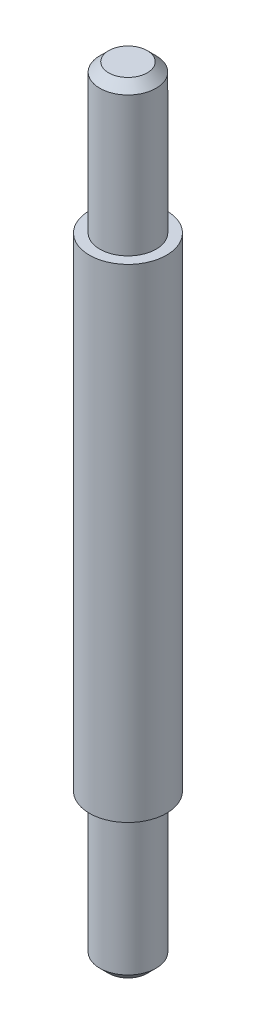
from build123d import *

# Parameters (mm, degrees)
END_CHAMFERS_3X45_SIZE = 3


with BuildPart() as part:
    # Pin Profile Sketch → Pin Body Revolve (revolve)
    with BuildSketch(Plane.XY, mode=Mode.PRIVATE) as pin_body_revolve_sk:
        Polygon((0, 131.5), (9.5, 131.5), (9.5, 81.5), (13, 81.5), (13, -81.5), (9.5, -81.5), (9.5, -131.5), (0, -131.5), align=None)
    revolve(pin_body_revolve_sk.sketch.rotate(Axis((0, 65.559405941, 0), (0, -1, 0)), 90), axis=Axis((0, 65.559405941, 0), (0, -1, 0)))

    # End Chamfers 3x45°
    end_chamfers_3x45_edges = [part.edges().sort_by_distance(p)[0] for p in [
        (0, -131.5, -9.5),
        (0, 131.5, -9.5),
    ]]
    chamfer(end_chamfers_3x45_edges, length=END_CHAMFERS_3X45_SIZE)


solid = part.part
